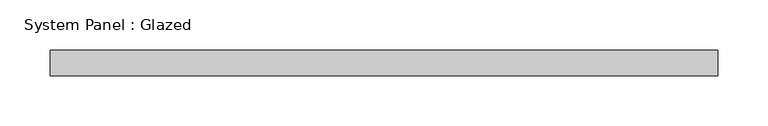
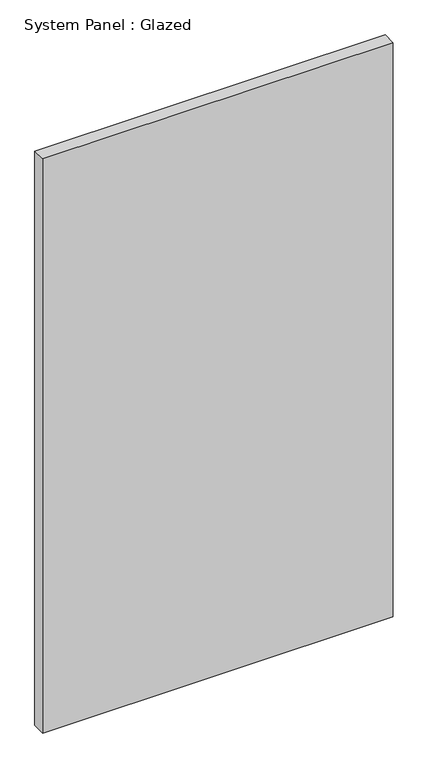
"""IFC4 building model written with IfcOpenShell, lengths in millimetres: plate geometry, System Panel : Glazed."""

from ifc_helpers import new_model, si_unit, origin, origin_with_axes, place, context, project, spatial, polyline, outline, extrude, source, transform, mapped, element, save


def system_panel_glazed_a4d37703(model_context):
    return source(origin(), model_context, "Body", "SweptSolid", [
        extrude(outline(polyline([(333.375, 19.05), (-333.375, 19.05), (-333.375, 44.45), (333.375, 44.45), (333.375, 19.05)])), origin_with_axes(), (0.0, 0.0, 1.0), 1154.4606784),
    ])


if __name__ == "__main__":
    model = new_model("IFC4")
    model_context = context("Model", 3, world=origin())
    ifc_project = project(units=[si_unit("LENGTHUNIT", "METRE", prefix="MILLI")], contexts=[model_context])
    site = spatial("IfcSite", under=ifc_project)
    building = spatial("IfcBuilding", under=site)
    placement = place(None, origin())
    system_panel_glazed_shape = system_panel_glazed_a4d37703(model_context)
    element("IfcPlate", 1, ObjectType="System Panel : Glazed", at=placement, inside=building, context=model_context, shape_type="MappedRepresentation", body=[
        mapped(system_panel_glazed_shape, transform((0.0, 0.0, 0.0), x_axis=(1.0, 0.0, 0.0), y_axis=(0.0, 1.0, 0.0), z_axis=(0.0, 0.0, 1.0))),
    ])
    save(model, "model.ifc")

# Revit data of these elements
# Type "System Panel : Glazed"
#   Construction Type Id = "GSP4R"
#   Analytic Construction = "1/8 in Pilkington single glazing"
#   Visual Light Transmittance = 0.9
#   Solar Heat Gain Coefficient = 0.86
#   Heat Transfer Coefficient (U) = 1.18115 BTU/(h·ft²·°F)
#   Define Thermal Properties by = 1
# Element 1 (IfcPlate, "System Panel : Glazed")
#   Materials on its faces: "Glass"
# Materials
#   "Glass": class "Glass", colour RGB 0 128 192, transparency 0.75, Description = "Soda Lime Glass", Cost = 0
